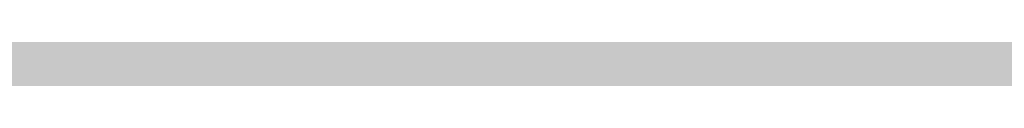
# Model space of a CAD drawing. Units: millimetres. Extents: x 0 to 2267, y 0 to 1823.
# Tile 179 of 256: x 1838.83 to 1841.442, y 1127.306 to 1127.384. Entities that reach past the tile are written whole.
import ezdxf

# ---------------------------------------------------------------- set-up
doc = ezdxf.new("R2010")
doc.units = ezdxf.units.MM
doc.header["$MEASUREMENT"] = 0
doc.layers.add('M-DIMS', color=2, linetype='Continuous', lineweight=25)
doc.layers.add('M-HATC', color=252, linetype='Continuous', lineweight=18)
doc.styles.get("Standard").update_dxf_attribs({"font": 'arial.ttf'})
doc.dimstyles.get("Standard").update_dxf_attribs({"dimtxt": 7, "dimasz": 4, "dimexe": 0.18, "dimexo": 0.0625, "dimgap": 0.09, "dimtad": 0, "dimdec": 0, "dimzin": 0, "dimdsep": 46, "dimtxsty": 'Standard', "dimcen": 0.09, "dimadec": 0, "dimazin": 0, "dimtfac": 1, "dimtdec": 0, "dimtofl": 0, "dimtmove": 0, "dimatfit": 3, "dimfxl": 1, "dimtolj": 1, "dimtzin": 0, "dimarcsym": 0})

# ---------------------------------------------------------------- blocks, each defined once
blk = doc.blocks.new('*D1')
at = {"layer": 'Defpoints', "color": 0, "transparency": 16777216}
for p in [(1593.4289, 1127.4171), (1843.4289, 1127.4171), (1843.4289, 955.6278)]:
    blk.add_point(p, dxfattribs=at)
at = {"layer": 'M-DIMS', "color": 0, "lineweight": -2, "transparency": 16777216}
for p, q in [((1593.4289, 1127.3546), (1593.4289, 955.4478)), ((1843.4289, 1127.3546), (1843.4289, 955.4478)), ((1597.4289, 955.6278), (1710.5582, 955.6278)), ((1839.4289, 955.6278), (1726.2996, 955.6278))]:
    blk.add_line(p, q, dxfattribs=at)
at = {"layer": 'M-DIMS', "color": 0, "transparency": 16777216}
for points in [[(1597.4289, 956.2944), (1597.4289, 954.9611), (1593.4289, 955.6278)], [(1839.4289, 956.2944), (1839.4289, 954.9611), (1843.4289, 955.6278)]]:
    blk.add_solid(points, dxfattribs=at)
at = {"layer": 'M-DIMS', "color": 0, "transparency": 16777216, "insert": (1718.4289, 955.6278), "char_height": 7, "attachment_point": 5}
blk.add_mtext('\\A1;250', dxfattribs=at)

msp = doc.modelspace()

# ---------------------------------------------------------------- hatches: boundary and pattern name
at = {"layer": 'M-HATC'}
h = msp.add_hatch(color=256, dxfattribs=at)
h.dxf.hatch_style = 1
h.paths.add_polyline_path([(2055.771, 1603.062), (1381.0868, 1603.062), (1381.0868, 1598.062), (2055.771, 1598.062)])
h.paths.add_polyline_path([(2055.771, 1598.062), (1381.0868, 1598.062), (1381.0868, 1593.062), (2055.771, 1593.062)])
h.paths.add_polyline_path([(2051.3074, 1536.7609), (1385.5504, 1536.7609), (1385.5504, 1526.7609), (1387.5504, 1526.7609), (1388.5366, 1525.0528), (1385.3319, 1521.2335), (1385.3319, 1521.2226), (2050.2542, 1522.7491), (2048.3212, 1525.0528), (2049.3074, 1526.7609), (2051.3074, 1526.7609)])
edge = h.paths.add_edge_path()
edge.add_arc((1847.5345, 1379.1492), 135, 222.603061, 222.890851, ccw=False)
edge.add_line((1748.1663, 1287.7656), (1683.0921, 1287.7656))
edge.add_arc((1583.7239, 1379.1492), 135, 317.109149, 317.396939, ccw=False)
edge.add_arc((1678.9686, 1290.6707), 5, 222.8909, 317.1091, ccw=False)
edge.add_arc((1774.2133, 1379.1492), 135, 222.603061, 222.890851, ccw=False)
edge.add_line((1674.8451, 1287.7656), (1609.7709, 1287.7656))
edge.add_arc((1510.4027, 1379.1492), 135, 317.109149, 317.396939, ccw=False)
edge.add_arc((1605.6474, 1290.6707), 5, 222.8909, 317.1091, ccw=False)
edge.add_arc((1700.8921, 1379.1492), 135, 222.603061, 222.890851, ccw=False)
edge.add_line((1601.5239, 1287.7656), (1536.4497, 1287.7656))
edge.add_arc((1437.0815, 1379.1492), 135, 317.109149, 317.396939, ccw=False)
edge.add_arc((1532.3262, 1290.6707), 5, 222.8909, 317.1091, ccw=False)
edge.add_arc((1627.5709, 1379.1492), 135, 222.603061, 222.890851, ccw=False)
edge.add_line((1528.2027, 1287.7656), (1505.9289, 1287.7656))
edge.add_spline(control_points=[(1505.9289, 1287.7656), (1504.2622, 1287.7656), (1504.2622, 1282.7656), (1505.9289, 1282.7656)], knot_values=[0, 0, 0, 0, 5, 5, 5, 5], degree=3, periodic=0)
edge.add_line((1505.9289, 1282.7656), (1930.9289, 1282.7656))
edge.add_spline(control_points=[(1930.9289, 1282.7656), (1932.5956, 1282.7656), (1932.5956, 1287.7656), (1930.9289, 1287.7656)], knot_values=[0, 0, 0, 0, 5, 5, 5, 5], degree=3, periodic=0)
edge.add_line((1930.9289, 1287.7656), (1903.0557, 1287.7656))
edge.add_arc((1803.6875, 1379.1492), 135, 317.109149, 317.396939, ccw=False)
edge.add_arc((1898.9322, 1290.6707), 5, 222.8909, 317.1091, ccw=False)
edge.add_arc((1994.1769, 1379.1492), 135, 222.603061, 222.890851, ccw=False)
edge.add_line((1894.8087, 1287.7656), (1829.7345, 1287.7656))
edge.add_arc((1730.3663, 1379.1492), 135, 317.109149, 317.396939, ccw=False)
edge.add_arc((1825.611, 1290.6707), 5, 222.8909, 317.1091, ccw=False)
edge.add_arc((1920.8557, 1379.1492), 135, 222.603061, 222.890851, ccw=False)
edge.add_line((1821.4875, 1287.7656), (1756.4133, 1287.7656))
edge.add_arc((1657.0451, 1379.1492), 135, 317.109149, 317.396939, ccw=False)
edge.add_arc((1752.2898, 1290.6707), 5, 222.8909, 317.1091, ccw=False)
edge = h.paths.add_edge_path()
edge.add_spline(control_points=[(1843.4289, 1227.2475), (1845.0956, 1227.2475), (1845.0956, 1232.2475), (1843.4289, 1232.2475)], knot_values=[0, 0, 0, 0, 5, 5, 5, 5], degree=3, periodic=0)
edge.add_line((1843.4289, 1232.2475), (1593.4289, 1232.2475))
edge.add_spline(control_points=[(1593.4289, 1232.2475), (1591.7622, 1232.2475), (1591.7622, 1227.2475), (1593.4289, 1227.2475)], knot_values=[0, 0, 0, 0, 5, 5, 5, 5], degree=3, periodic=0)
edge.add_line((1593.4289, 1227.2475), (1843.4289, 1227.2475))
h.paths.add_polyline_path([(1905.9289, 1127.4171), (1530.9289, 1127.4171, 0.414214), (1520.9289, 1117.4171), (1530.9289, 1117.4171), (1915.9289, 1117.4171, 0.414214)])
edge = h.paths.add_edge_path()
edge.add_arc((1397.0858, 1498.4078), 12.7299, 90.78215, 190.87871, ccw=False)
edge.add_line((1396.912, 1511.1365), (1428.0097, 1511.3488))
edge.add_line((1428.0097, 1511.3488), (1433.0097, 1511.3488))
edge.add_line((1433.0097, 1511.3488), (1434.439, 1511.3488))
edge.add_arc((1419.474, 1498.0804), 20, 41.561, 74.08211)
edge.add_line((1424.9592, 1517.3135), (1399.9351, 1517.2561))
edge.add_spline(control_points=[(1399.9307, 1517.2561), (1399.884, 1517.2131), (1399.8328, 1517.1689), (1399.7774, 1517.1236)], knot_values=[11.567499, 11.567499, 11.567499, 11.567499, 11.814249, 11.814249, 11.814249, 11.814249], degree=3, periodic=0)
edge.add_spline(control_points=[(1399.6328, 1517.0099), (1399.5831, 1516.9721), (1399.5307, 1516.9338), (1399.4759, 1516.8947)], knot_values=[11.167718, 11.167718, 11.167718, 11.167718, 11.365188, 11.365188, 11.365188, 11.365188], degree=3, periodic=0)
edge.add_spline(control_points=[(1399.3398, 1516.8001), (1399.1514, 1516.6719), (1398.9384, 1516.5377), (1398.704, 1516.3994)], knot_values=[10.376405, 10.376405, 10.376405, 10.376405, 11.00994, 11.00994, 11.00994, 11.00994], degree=3, periodic=0)
edge.add_spline(control_points=[(1398.6572, 1516.3719), (1398.5789, 1516.326), (1398.4983, 1516.2797), (1398.4155, 1516.2331)], knot_values=[10.125175, 10.125175, 10.125175, 10.125175, 10.334406, 10.334406, 10.334406, 10.334406], degree=3, periodic=0)
edge.add_spline(control_points=[(1398.2642, 1516.1487), (1398.196, 1516.1111), (1398.1263, 1516.0732), (1398.0555, 1516.0351)], knot_values=[9.832246, 9.832246, 9.832246, 9.832246, 9.999658, 9.999658, 9.999658, 9.999658], degree=3, periodic=0)
edge.add_spline(control_points=[(1397.9987, 1516.0048), (1397.7312, 1515.8621), (1397.446, 1515.7171), (1397.1466, 1515.5714)], knot_values=[9.161808, 9.161808, 9.161808, 9.161808, 9.787769, 9.787769, 9.787769, 9.787769], degree=3, periodic=0)
edge.add_spline(control_points=[(1397.1466, 1515.5714), (1396.8418, 1515.423), (1396.5222, 1515.274), (1396.1914, 1515.1262)], knot_values=[8.524455, 8.524455, 8.524455, 8.524455, 9.161808, 9.161808, 9.161808, 9.161808], degree=3, periodic=0)
edge.add_spline(control_points=[(1396.0777, 1515.0756), (1395.9854, 1515.0348), (1395.8922, 1514.994), (1395.7983, 1514.9534)], knot_values=[8.275193, 8.275193, 8.275193, 8.275193, 8.451726, 8.451726, 8.451726, 8.451726], degree=3, periodic=0)
edge.add_spline(control_points=[(1395.6018, 1514.8691), (1395.4997, 1514.8257), (1395.3968, 1514.7824), (1395.2932, 1514.7394)], knot_values=[7.962917, 7.962917, 7.962917, 7.962917, 8.152764, 8.152764, 8.152764, 8.152764], degree=3, periodic=0)
edge.add_spline(control_points=[(1395.2116, 1514.7057), (1394.8278, 1514.5475), (1394.4345, 1514.3929), (1394.0364, 1514.2442)], knot_values=[7.21254, 7.21254, 7.21254, 7.21254, 7.913148, 7.913148, 7.913148, 7.913148], degree=3, periodic=0)
edge.add_spline(control_points=[(1394.0364, 1514.2442), (1393.7076, 1514.1214), (1393.3754, 1514.0027), (1393.0427, 1513.8895)], knot_values=[6.633733, 6.633733, 6.633733, 6.633733, 7.21254, 7.21254, 7.21254, 7.21254], degree=3, periodic=0)
edge.add_spline(control_points=[(1392.8214, 1513.815), (1392.7198, 1513.7812), (1392.6181, 1513.7479), (1392.5166, 1513.7152)], knot_values=[6.328796, 6.328796, 6.328796, 6.328796, 6.505493, 6.505493, 6.505493, 6.505493], degree=3, periodic=0)
edge.add_spline(control_points=[(1392.5166, 1513.7152), (1392.3187, 1513.6515), (1392.1212, 1513.59), (1391.9244, 1513.531)], knot_values=[5.984605, 5.984605, 5.984605, 5.984605, 6.328796, 6.328796, 6.328796, 6.328796], degree=3, periodic=0)
edge.add_spline(control_points=[(1391.7915, 1513.4915), (1391.3122, 1513.3501), (1390.8384, 1513.2239), (1390.3784, 1513.1171)], knot_values=[5.066697, 5.066697, 5.066697, 5.066697, 5.907055, 5.907055, 5.907055, 5.907055], degree=3, periodic=0)
edge.add_spline(control_points=[(1390.3784, 1513.1171), (1390.1797, 1513.071), (1389.9836, 1513.0284), (1389.7907, 1512.9899)], knot_values=[4.70367, 4.70367, 4.70367, 4.70367, 5.066695, 5.066695, 5.066695, 5.066695], degree=3, periodic=0)
edge.add_spline(control_points=[(1389.422, 1512.9204), (1389.2459, 1512.8892), (1389.0729, 1512.8617), (1388.9036, 1512.8381)], knot_values=[4.130571, 4.130571, 4.130571, 4.130571, 4.469816, 4.469816, 4.469816, 4.469816], degree=3, periodic=0)
edge.add_spline(control_points=[(1388.9036, 1512.8381), (1388.591, 1512.7946), (1388.2911, 1512.7644), (1388.0071, 1512.7494)], knot_values=[3.504031, 3.504031, 3.504031, 3.504031, 4.130571, 4.130571, 4.130571, 4.130571], degree=3, periodic=0)
edge.add_spline(control_points=[(1387.9356, 1512.7459), (1387.8538, 1512.7423), (1387.7733, 1512.74), (1387.6944, 1512.739)], knot_values=[3.268866, 3.268866, 3.268866, 3.268866, 3.451164, 3.451164, 3.451164, 3.451164], degree=3, periodic=0)
edge.add_spline(control_points=[(1387.3351, 1512.7443), (1387.2076, 1512.7499), (1387.0847, 1512.7597), (1386.967, 1512.7739)], knot_values=[2.670686, 2.670686, 2.670686, 2.670686, 2.984, 2.984, 2.984, 2.984], degree=3, periodic=0)
edge.add_spline(control_points=[(1386.8327, 1512.7922), (1386.8209, 1512.7941), (1386.8092, 1512.7959), (1386.7975, 1512.7979)], knot_values=[2.516981, 2.516981, 2.516981, 2.516981, 2.549528, 2.549528, 2.549528, 2.549528], degree=3, periodic=0)
edge.add_spline(control_points=[(1386.4526, 1512.8735), (1386.4257, 1512.881), (1386.3993, 1512.889), (1386.3733, 1512.8972)], knot_values=[2.095869, 2.095869, 2.095869, 2.095869, 2.17941, 2.17941, 2.17941, 2.17941], degree=3, periodic=0)
edge.add_spline(control_points=[(1386.0691, 1513.0189), (1386.0634, 1513.0217), (1386.0577, 1513.0246), (1386.052, 1513.0275)], knot_values=[1.72453, 1.72453, 1.72453, 1.72453, 1.745933, 1.745933, 1.745933, 1.745933], degree=3, periodic=0)
edge.add_arc((1399.474, 1498.0804), 20, 131.82432, 180)
edge.add_arc((1630.3336, 1505.5484), 250.9708, 181.705176, 236.427975)
edge.add_arc((1605.3399, 1483.3044), 218.7822, 238.660829, 243.34961)
edge.add_arc((1647.0911, 1510.3592), 262.8986, 183.129836, 237.853442, ccw=False)
h.paths.add_polyline_path([(1406.5369, 1391.9644, 0.149382), (1491.5506, 1296.4418, -0.129517)], flags=17)
edge = h.paths.add_edge_path()
edge.add_arc((2037.3838, 1498.0804), 20, 0, 48.26587)
edge.add_spline(control_points=[(2050.6973, 1513.0052), (2050.6512, 1512.9847), (2050.6034, 1512.9655), (2050.5539, 1512.9477)], knot_values=[1.835652, 1.835652, 1.835652, 1.835652, 2.000781, 2.000781, 2.000781, 2.000781], degree=3, periodic=0)
edge.add_spline(control_points=[(2050.4616, 1512.9166), (2050.479, 1512.9221), (2050.4963, 1512.9277), (2050.5133, 1512.9335)], knot_values=[2.045477, 2.045477, 2.045477, 2.045477, 2.101389, 2.101389, 2.101389, 2.101389], degree=3, periodic=0)
edge.add_spline(control_points=[(2050.129, 1512.8342), (2050.1984, 1512.8473), (2050.2657, 1512.8623), (2050.3308, 1512.8792)], knot_values=[2.237629, 2.237629, 2.237629, 2.237629, 2.435841, 2.435841, 2.435841, 2.435841], degree=3, periodic=0)
edge.add_spline(control_points=[(2050.0946, 1512.8278), (2050.1061, 1512.8299), (2050.1176, 1512.832), (2050.129, 1512.8342)], knot_values=[2.435841, 2.435841, 2.435841, 2.435841, 2.468321, 2.468321, 2.468321, 2.468321], degree=3, periodic=0)
edge.add_spline(control_points=[(2049.7843, 1512.7851), (2049.8552, 1512.7922), (2049.9243, 1512.8008), (2049.9917, 1512.8109)], knot_values=[2.563852, 2.563852, 2.563852, 2.563852, 2.748541, 2.748541, 2.748541, 2.748541], degree=3, periodic=0)
edge.add_spline(control_points=[(2049.4052, 1512.7617), (2049.5364, 1512.7653), (2049.6629, 1512.773), (2049.7843, 1512.7851)], knot_values=[2.748541, 2.748541, 2.748541, 2.748541, 3.064882, 3.064882, 3.064882, 3.064882], degree=3, periodic=0)
edge.add_spline(control_points=[(2049.1698, 1512.7597), (2049.2336, 1512.7591), (2049.2965, 1512.7594), (2049.3584, 1512.7606)], knot_values=[3.102309, 3.102309, 3.102309, 3.102309, 3.2503, 3.2503, 3.2503, 3.2503], degree=3, periodic=0)
edge.add_spline(control_points=[(2048.8573, 1512.7691), (2048.9638, 1512.7638), (2049.068, 1512.7606), (2049.1698, 1512.7597)], knot_values=[3.2503, 3.2503, 3.2503, 3.2503, 3.486069, 3.486069, 3.486069, 3.486069], degree=3, periodic=0)
edge.add_spline(control_points=[(2048.6924, 1512.7789), (2048.3729, 1512.8009), (2048.0345, 1512.8411), (2047.6817, 1512.897)], knot_values=[3.606429, 3.606429, 3.606429, 3.606429, 4.2989, 4.2989, 4.2989, 4.2989], degree=3, periodic=0)
edge.add_spline(control_points=[(2047.6817, 1512.897), (2047.5458, 1512.9185), (2047.4077, 1512.9424), (2047.2678, 1512.9685)], knot_values=[4.2989, 4.2989, 4.2989, 4.2989, 4.565769, 4.565769, 4.565769, 4.565769], degree=3, periodic=0)
edge.add_spline(control_points=[(2047.2678, 1512.9685), (2047.1449, 1512.9914), (2047.0207, 1513.016), (2046.8951, 1513.0422)], knot_values=[4.565769, 4.565769, 4.565769, 4.565769, 4.799971, 4.799971, 4.799971, 4.799971], degree=3, periodic=0)
edge.add_spline(control_points=[(2046.8951, 1513.0422), (2046.5286, 1513.1188), (2046.1513, 1513.209), (2045.7676, 1513.3107)], knot_values=[4.799971, 4.799971, 4.799971, 4.799971, 5.483718, 5.483718, 5.483718, 5.483718], degree=3, periodic=0)
edge.add_spline(control_points=[(2045.7676, 1513.3107), (2045.3724, 1513.4154), (2044.9704, 1513.5322), (2044.5662, 1513.6588)], knot_values=[5.483718, 5.483718, 5.483718, 5.483718, 6.187866, 6.187866, 6.187866, 6.187866], degree=3, periodic=0)
edge.add_spline(control_points=[(2044.5662, 1513.6588), (2044.4149, 1513.7061), (2044.2633, 1513.7549), (2044.1116, 1513.8048)], knot_values=[6.187866, 6.187866, 6.187866, 6.187866, 6.451551, 6.451551, 6.451551, 6.451551], degree=3, periodic=0)
edge.add_spline(control_points=[(2044.1116, 1513.8048), (2043.9967, 1513.8427), (2043.8817, 1513.8813), (2043.7668, 1513.9205)], knot_values=[6.451551, 6.451551, 6.451551, 6.451551, 6.651434, 6.651434, 6.651434, 6.651434], degree=3, periodic=0)
edge.add_spline(control_points=[(2043.7668, 1513.9205), (2043.3716, 1514.0554), (2042.9774, 1514.1979), (2042.5886, 1514.3458)], knot_values=[6.651434, 6.651434, 6.651434, 6.651434, 7.338879, 7.338879, 7.338879, 7.338879], degree=3, periodic=0)
edge.add_spline(control_points=[(2042.5886, 1514.3458), (2042.1643, 1514.5071), (2041.7465, 1514.6749), (2041.3409, 1514.846)], knot_values=[7.338879, 7.338879, 7.338879, 7.338879, 8.089209, 8.089209, 8.089209, 8.089209], degree=3, periodic=0)
edge.add_spline(control_points=[(2041.3409, 1514.846), (2041.1028, 1514.9465), (2040.869, 1515.0481), (2040.6405, 1515.1502)], knot_values=[8.089209, 8.089209, 8.089209, 8.089209, 8.529587, 8.529587, 8.529587, 8.529587], degree=3, periodic=0)
edge.add_spline(control_points=[(2040.51, 1515.2089), (2040.0824, 1515.4022), (2039.6747, 1515.5971), (2039.295, 1515.7894)], knot_values=[8.613818, 8.613818, 8.613818, 8.613818, 9.44571, 9.44571, 9.44571, 9.44571], degree=3, periodic=0)
edge.add_spline(control_points=[(2039.295, 1515.7894), (2039.0618, 1515.9075), (2038.8391, 1516.0246), (2038.6288, 1516.1398)], knot_values=[9.44571, 9.44571, 9.44571, 9.44571, 9.956404, 9.956404, 9.956404, 9.956404], degree=3, periodic=0)
edge.add_spline(control_points=[(2038.6288, 1516.1398), (2038.5187, 1516.2001), (2038.4121, 1516.2598), (2038.309, 1516.3189)], knot_values=[9.956404, 9.956404, 9.956404, 9.956404, 10.223542, 10.223542, 10.223542, 10.223542], degree=3, periodic=0)
edge.add_spline(control_points=[(2038.309, 1516.3189), (2038.2138, 1516.3735), (2038.1216, 1516.4276), (2038.0328, 1516.481)], knot_values=[10.223542, 10.223542, 10.223542, 10.223542, 10.47051, 10.47051, 10.47051, 10.47051], degree=3, periodic=0)
edge.add_spline(control_points=[(2038.0328, 1516.481), (2037.7855, 1516.6296), (2037.5639, 1516.773), (2037.3722, 1516.909)], knot_values=[10.47051, 10.47051, 10.47051, 10.47051, 11.15767, 11.15767, 11.15767, 11.15767], degree=3, periodic=0)
edge.add_spline(control_points=[(2037.3722, 1516.909), (2037.2789, 1516.9752), (2037.1927, 1517.0396), (2037.1142, 1517.102)], knot_values=[11.15767, 11.15767, 11.15767, 11.15767, 11.49227, 11.49227, 11.49227, 11.49227], degree=3, periodic=0)
edge.add_spline(control_points=[(2036.8564, 1517.3259), (2036.9148, 1517.2692), (2036.9814, 1517.2103), (2037.0557, 1517.1492)], knot_values=[11.577341, 11.577341, 11.577341, 11.577341, 11.91035, 11.91035, 11.91035, 11.91035], degree=3, periodic=0)
edge.add_spline(control_points=[(2036.8074, 1517.3748), (2036.823, 1517.3587), (2036.8393, 1517.3424), (2036.8564, 1517.3259)], knot_values=[11.91035, 11.91035, 11.91035, 11.91035, 12.007402, 12.007402, 12.007402, 12.007402], degree=3, periodic=0)
edge.add_spline(control_points=[(2036.7017, 1517.494), (2036.7104, 1517.483), (2036.7196, 1517.4719), (2036.7291, 1517.4606)], knot_values=[12.184155, 12.184155, 12.184155, 12.184155, 12.255409, 12.255409, 12.255409, 12.255409], degree=3, periodic=0)
edge.add_spline(control_points=[(2036.6159, 1517.6205), (2036.62, 1517.613), (2036.6243, 1517.6055), (2036.6289, 1517.5979)], knot_values=[12.487913, 12.487913, 12.487913, 12.487913, 12.541035, 12.541035, 12.541035, 12.541035], degree=3, periodic=0)
edge.add_spline(control_points=[(2036.5635, 1517.786), (2036.5637, 1517.7794), (2036.5642, 1517.7726), (2036.565, 1517.7658)], knot_values=[12.911761, 12.911761, 12.911761, 12.911761, 12.968286, 12.968286, 12.968286, 12.968286], degree=3, periodic=0)
edge.add_spline(control_points=[(2036.6166, 1517.9304), (2036.6125, 1517.9259), (2036.6086, 1517.9212), (2036.6049, 1517.9165)], knot_values=[13.382527, 13.382527, 13.382527, 13.382527, 13.433791, 13.433791, 13.433791, 13.433791], degree=3, periodic=0)
edge.add_spline(control_points=[(2036.749, 1518.017), (2036.7361, 1518.0116), (2036.7239, 1518.006), (2036.7124, 1518.0002)], knot_values=[13.726299, 13.726299, 13.726299, 13.726299, 13.809928, 13.809928, 13.809928, 13.809928], degree=3, periodic=0)
edge.add_spline(control_points=[(2036.8604, 1518.0528), (2036.8386, 1518.0474), (2036.8181, 1518.0416), (2036.7988, 1518.0353)], knot_values=[13.910887, 13.910887, 13.910887, 13.910887, 14.02153, 14.02153, 14.02153, 14.02153], degree=3, periodic=0)
edge.add_line((2036.9639, 1518.0804), (2032.3838, 1518.0804))
edge.add_line((2032.3838, 1518.0804), (2027.3838, 1518.0804))
edge.add_line((2027.3838, 1518.0804), (2022.3838, 1518.0804))
edge.add_line((2022.3838, 1518.0804), (2017.3838, 1518.0804))
edge.add_arc((2017.3838, 1498.0804), 20, 90, 138.439)
edge.add_line((2002.4188, 1511.3488), (2003.8481, 1511.3488))
edge.add_line((2003.8481, 1511.3488), (2008.8481, 1511.3488))
edge.add_line((2008.8481, 1511.3488), (2039.772, 1511.1377))
edge.add_arc((2039.772, 1498.4078), 12.7299, -10.87871, 90, ccw=False)
edge.add_arc((1789.7668, 1510.3592), 262.8986, 302.146558, 356.870164, ccw=False)
edge.add_arc((1831.5179, 1483.3044), 218.7822, 296.65039, 301.339171)
edge.add_arc((1806.5242, 1505.5484), 250.9708, 303.572025, 358.294824)
h.paths.add_polyline_path([(2030.321, 1391.9644, -0.129517), (1945.3072, 1296.4418, 0.149382)], flags=17)
edge = h.paths.add_edge_path()
edge.add_spline(control_points=[(2037.2464, 1518.0821), (2037.2898, 1518.081), (2037.3355, 1518.0804), (2037.3838, 1518.0804)], knot_values=[0.000012, 0.000012, 0.000012, 0.000012, 0.144754, 0.144754, 0.144754, 0.144754], degree=3, periodic=0)
edge.add_line((2037.3357, 1518.0804), (2037.0096, 1518.0804))
edge.add_spline(control_points=[(2037.0096, 1518.0804), (2036.9822, 1518.0768), (2036.956, 1518.0727), (2036.9312, 1518.0681)], knot_values=[14.13465, 14.13465, 14.13465, 14.13465, 14.247197, 14.247197, 14.247197, 14.247197], degree=3, periodic=0)
edge.add_spline(control_points=[(2036.9312, 1518.0681), (2036.9276, 1518.0674), (2036.9241, 1518.0667), (2036.9205, 1518.0661)], knot_values=[14.118315, 14.118315, 14.118315, 14.118315, 14.13465, 14.13465, 14.13465, 14.13465], degree=3, periodic=0)
edge.add_spline(control_points=[(2036.9205, 1518.0661), (2036.9118, 1518.0644), (2036.9032, 1518.0626), (2036.8948, 1518.0608)], knot_values=[14.078086, 14.078086, 14.078086, 14.078086, 14.118315, 14.118315, 14.118315, 14.118315], degree=3, periodic=0)
edge.add_spline(control_points=[(2036.8948, 1518.0608), (2036.883, 1518.0583), (2036.8716, 1518.0556), (2036.8604, 1518.0528)], knot_values=[14.02153, 14.02153, 14.02153, 14.02153, 14.078086, 14.078086, 14.078086, 14.078086], degree=3, periodic=0)
edge.add_spline(control_points=[(2036.8604, 1518.0528), (2036.8386, 1518.0474), (2036.8181, 1518.0416), (2036.7988, 1518.0353)], knot_values=[13.910887, 13.910887, 13.910887, 13.910887, 14.02153, 14.02153, 14.02153, 14.02153], degree=3, periodic=0)
edge.add_spline(control_points=[(2036.7988, 1518.0353), (2036.7981, 1518.035), (2036.7974, 1518.0348), (2036.7967, 1518.0346)], knot_values=[13.906906, 13.906906, 13.906906, 13.906906, 13.910887, 13.910887, 13.910887, 13.910887], degree=3, periodic=0)
edge.add_spline(control_points=[(2036.7967, 1518.0346), (2036.7882, 1518.0318), (2036.7799, 1518.0289), (2036.7719, 1518.0259)], knot_values=[13.857826, 13.857826, 13.857826, 13.857826, 13.906906, 13.906906, 13.906906, 13.906906], degree=3, periodic=0)
edge.add_spline(control_points=[(2036.7719, 1518.0259), (2036.764, 1518.023), (2036.7564, 1518.02), (2036.749, 1518.017)], knot_values=[13.809928, 13.809928, 13.809928, 13.809928, 13.857826, 13.857826, 13.857826, 13.857826], degree=3, periodic=0)
edge.add_spline(control_points=[(2036.749, 1518.017), (2036.7361, 1518.0116), (2036.7239, 1518.006), (2036.7124, 1518.0002)], knot_values=[13.726299, 13.726299, 13.726299, 13.726299, 13.809928, 13.809928, 13.809928, 13.809928], degree=3, periodic=0)
edge.add_spline(control_points=[(2036.7124, 1518.0002), (2036.7121, 1518), (2036.7118, 1517.9999), (2036.7115, 1517.9997)], knot_values=[13.723993, 13.723993, 13.723993, 13.723993, 13.726299, 13.726299, 13.726299, 13.726299], degree=3, periodic=0)
edge.add_spline(control_points=[(2036.7115, 1517.9997), (2036.7063, 1517.9971), (2036.7013, 1517.9944), (2036.6965, 1517.9917)], knot_values=[13.686536, 13.686536, 13.686536, 13.686536, 13.723993, 13.723993, 13.723993, 13.723993], degree=3, periodic=0)
edge.add_spline(control_points=[(2036.6965, 1517.9917), (2036.6919, 1517.9891), (2036.6874, 1517.9865), (2036.6831, 1517.9839)], knot_values=[13.651251, 13.651251, 13.651251, 13.651251, 13.686536, 13.686536, 13.686536, 13.686536], degree=3, periodic=0)
edge.add_spline(control_points=[(2036.6831, 1517.9839), (2036.6764, 1517.9798), (2036.67, 1517.9757), (2036.6639, 1517.9714)], knot_values=[13.596804, 13.596804, 13.596804, 13.596804, 13.651251, 13.651251, 13.651251, 13.651251], degree=3, periodic=0)
edge.add_spline(control_points=[(2036.6639, 1517.9714), (2036.6636, 1517.9712), (2036.6633, 1517.9709), (2036.6629, 1517.9707)], knot_values=[13.593956, 13.593956, 13.593956, 13.593956, 13.596804, 13.596804, 13.596804, 13.596804], degree=3, periodic=0)
edge.add_spline(control_points=[(2036.6629, 1517.9707), (2036.6603, 1517.9689), (2036.6577, 1517.967), (2036.6552, 1517.9651)], knot_values=[13.570322, 13.570322, 13.570322, 13.570322, 13.593956, 13.593956, 13.593956, 13.593956], degree=3, periodic=0)
edge.add_spline(control_points=[(2036.6552, 1517.9651), (2036.6525, 1517.9631), (2036.6499, 1517.9611), (2036.6474, 1517.9591)], knot_values=[13.545477, 13.545477, 13.545477, 13.545477, 13.570322, 13.570322, 13.570322, 13.570322], degree=3, periodic=0)
edge.add_spline(control_points=[(2036.6474, 1517.9591), (2036.6472, 1517.9589), (2036.6471, 1517.9588), (2036.6469, 1517.9587)], knot_values=[13.543931, 13.543931, 13.543931, 13.543931, 13.545477, 13.545477, 13.545477, 13.545477], degree=3, periodic=0)
edge.add_spline(control_points=[(2036.6469, 1517.9587), (2036.6412, 1517.9541), (2036.6358, 1517.9494), (2036.6307, 1517.9447)], knot_values=[13.488237, 13.488237, 13.488237, 13.488237, 13.543931, 13.543931, 13.543931, 13.543931], degree=3, periodic=0)
edge.add_spline(control_points=[(2036.6307, 1517.9447), (2036.6282, 1517.9423), (2036.6257, 1517.9399), (2036.6233, 1517.9374)], knot_values=[13.460307, 13.460307, 13.460307, 13.460307, 13.488237, 13.488237, 13.488237, 13.488237], degree=3, periodic=0)
edge.add_spline(control_points=[(2036.6233, 1517.9374), (2036.6215, 1517.9356), (2036.6198, 1517.9338), (2036.6181, 1517.932)], knot_values=[13.439712, 13.439712, 13.439712, 13.439712, 13.460307, 13.460307, 13.460307, 13.460307], degree=3, periodic=0)
edge.add_spline(control_points=[(2036.6181, 1517.932), (2036.6176, 1517.9315), (2036.6171, 1517.9309), (2036.6166, 1517.9304)], knot_values=[13.433791, 13.433791, 13.433791, 13.433791, 13.439712, 13.439712, 13.439712, 13.439712], degree=3, periodic=0)
edge.add_spline(control_points=[(2036.6166, 1517.9304), (2036.6125, 1517.9259), (2036.6086, 1517.9212), (2036.6049, 1517.9165)], knot_values=[13.382527, 13.382527, 13.382527, 13.382527, 13.433791, 13.433791, 13.433791, 13.433791], degree=3, periodic=0)
edge.add_spline(control_points=[(2036.6049, 1517.9165), (2036.6026, 1517.9135), (2036.6004, 1517.9104), (2036.5982, 1517.9074)], knot_values=[13.350017, 13.350017, 13.350017, 13.350017, 13.382527, 13.382527, 13.382527, 13.382527], degree=3, periodic=0)
edge.add_spline(control_points=[(2036.5982, 1517.9074), (2036.5972, 1517.9059), (2036.5962, 1517.9043), (2036.5952, 1517.9028)], knot_values=[13.333922, 13.333922, 13.333922, 13.333922, 13.350017, 13.350017, 13.350017, 13.350017], degree=3, periodic=0)
edge.add_spline(control_points=[(2036.5952, 1517.9028), (2036.5945, 1517.9018), (2036.5939, 1517.9009), (2036.5933, 1517.8999)], knot_values=[13.323828, 13.323828, 13.323828, 13.323828, 13.333922, 13.333922, 13.333922, 13.333922], degree=3, periodic=0)
edge.add_spline(control_points=[(2036.5933, 1517.8999), (2036.5905, 1517.8955), (2036.5879, 1517.8909), (2036.5855, 1517.8864)], knot_values=[13.277545, 13.277545, 13.277545, 13.277545, 13.323828, 13.323828, 13.323828, 13.323828], degree=3, periodic=0)
edge.add_spline(control_points=[(2036.5855, 1517.8864), (2036.5836, 1517.8827), (2036.5817, 1517.8789), (2036.5801, 1517.8751)], knot_values=[13.240119, 13.240119, 13.240119, 13.240119, 13.277545, 13.277545, 13.277545, 13.277545], degree=3, periodic=0)
edge.add_spline(control_points=[(2036.5801, 1517.8751), (2036.5795, 1517.8739), (2036.579, 1517.8727), (2036.5785, 1517.8715)], knot_values=[13.228211, 13.228211, 13.228211, 13.228211, 13.240119, 13.240119, 13.240119, 13.240119], degree=3, periodic=0)
edge.add_spline(control_points=[(2036.5785, 1517.8715), (2036.578, 1517.8702), (2036.5774, 1517.869), (2036.5769, 1517.8677)], knot_values=[13.215717, 13.215717, 13.215717, 13.215717, 13.228211, 13.228211, 13.228211, 13.228211], degree=3, periodic=0)
edge.add_spline(control_points=[(2036.5769, 1517.8677), (2036.5755, 1517.864), (2036.5741, 1517.8603), (2036.5729, 1517.8565)], knot_values=[13.179847, 13.179847, 13.179847, 13.179847, 13.215717, 13.215717, 13.215717, 13.215717], degree=3, periodic=0)
edge.add_spline(control_points=[(2036.5729, 1517.8565), (2036.5713, 1517.8515), (2036.5699, 1517.8464), (2036.5687, 1517.8413)], knot_values=[13.132017, 13.132017, 13.132017, 13.132017, 13.179847, 13.179847, 13.179847, 13.179847], degree=3, periodic=0)
edge.add_spline(control_points=[(2036.5687, 1517.8413), (2036.5684, 1517.8402), (2036.5682, 1517.8392), (2036.568, 1517.8382)], knot_values=[13.122482, 13.122482, 13.122482, 13.122482, 13.132017, 13.132017, 13.132017, 13.132017], degree=3, periodic=0)
edge.add_spline(control_points=[(2036.568, 1517.8382), (2036.5676, 1517.8363), (2036.5672, 1517.8345), (2036.5669, 1517.8327)], knot_values=[13.105592, 13.105592, 13.105592, 13.105592, 13.122482, 13.122482, 13.122482, 13.122482], degree=3, periodic=0)
edge.add_spline(control_points=[(2036.5669, 1517.8327), (2036.5662, 1517.8292), (2036.5657, 1517.8257), (2036.5652, 1517.8222)], knot_values=[13.074063, 13.074063, 13.074063, 13.074063, 13.105592, 13.105592, 13.105592, 13.105592], degree=3, periodic=0)
edge.add_spline(control_points=[(2036.5652, 1517.8222), (2036.5652, 1517.8222), (2036.5652, 1517.8222), (2036.5652, 1517.8222)], knot_values=[13.074043, 13.074043, 13.074043, 13.074043, 13.074063, 13.074063, 13.074063, 13.074063], degree=3, periodic=0)
edge.add_spline(control_points=[(2036.5652, 1517.8222), (2036.5644, 1517.8164), (2036.5639, 1517.8106), (2036.5636, 1517.8046)], knot_values=[13.021884, 13.021884, 13.021884, 13.021884, 13.074043, 13.074043, 13.074043, 13.074043], degree=3, periodic=0)
edge.add_spline(control_points=[(2036.5636, 1517.8046), (2036.5636, 1517.804), (2036.5636, 1517.8034), (2036.5635, 1517.8028)], knot_values=[13.01674, 13.01674, 13.01674, 13.01674, 13.021884, 13.021884, 13.021884, 13.021884], degree=3, periodic=0)
edge.add_spline(control_points=[(2036.5635, 1517.8028), (2036.5634, 1517.8005), (2036.5634, 1517.7982), (2036.5634, 1517.7958)], knot_values=[12.996438, 12.996438, 12.996438, 12.996438, 13.01674, 13.01674, 13.01674, 13.01674], degree=3, periodic=0)
edge.add_spline(control_points=[(2036.5634, 1517.7958), (2036.5633, 1517.7926), (2036.5634, 1517.7893), (2036.5635, 1517.786)], knot_values=[12.968286, 12.968286, 12.968286, 12.968286, 12.996438, 12.996438, 12.996438, 12.996438], degree=3, periodic=0)
edge.add_spline(control_points=[(2036.5635, 1517.786), (2036.5637, 1517.7794), (2036.5642, 1517.7726), (2036.565, 1517.7658)], knot_values=[12.911761, 12.911761, 12.911761, 12.911761, 12.968286, 12.968286, 12.968286, 12.968286], degree=3, periodic=0)
edge.add_spline(control_points=[(2036.565, 1517.7658), (2036.565, 1517.7657), (2036.565, 1517.7656), (2036.565, 1517.7656)], knot_values=[12.911017, 12.911017, 12.911017, 12.911017, 12.911761, 12.911761, 12.911761, 12.911761], degree=3, periodic=0)
edge.add_spline(control_points=[(2036.565, 1517.7656), (2036.5654, 1517.7625), (2036.5658, 1517.7593), (2036.5663, 1517.7562)], knot_values=[12.88528, 12.88528, 12.88528, 12.88528, 12.911017, 12.911017, 12.911017, 12.911017], degree=3, periodic=0)
edge.add_spline(control_points=[(2036.5663, 1517.7562), (2036.5667, 1517.7534), (2036.5672, 1517.7506), (2036.5677, 1517.7478)], knot_values=[12.862519, 12.862519, 12.862519, 12.862519, 12.88528, 12.88528, 12.88528, 12.88528], degree=3, periodic=0)
edge.add_spline(control_points=[(2036.5677, 1517.7478), (2036.5678, 1517.7474), (2036.5679, 1517.7469), (2036.568, 1517.7465)], knot_values=[12.858885, 12.858885, 12.858885, 12.858885, 12.862519, 12.862519, 12.862519, 12.862519], degree=3, periodic=0)
edge.add_spline(control_points=[(2036.568, 1517.7465), (2036.5692, 1517.7399), (2036.5707, 1517.7332), (2036.5724, 1517.7264)], knot_values=[12.8053, 12.8053, 12.8053, 12.8053, 12.858885, 12.858885, 12.858885, 12.858885], degree=3, periodic=0)
edge.add_spline(control_points=[(2036.5724, 1517.7264), (2036.5734, 1517.7226), (2036.5745, 1517.7187), (2036.5756, 1517.7149)], knot_values=[12.775176, 12.775176, 12.775176, 12.775176, 12.8053, 12.8053, 12.8053, 12.8053], degree=3, periodic=0)
edge.add_spline(control_points=[(2036.5756, 1517.7149), (2036.5763, 1517.7125), (2036.577, 1517.7102), (2036.5778, 1517.7078)], knot_values=[12.756759, 12.756759, 12.756759, 12.756759, 12.775176, 12.775176, 12.775176, 12.775176], degree=3, periodic=0)
edge.add_spline(control_points=[(2036.5778, 1517.7078), (2036.5781, 1517.7067), (2036.5784, 1517.7057), (2036.5787, 1517.7047)], knot_values=[12.748742, 12.748742, 12.748742, 12.748742, 12.756759, 12.756759, 12.756759, 12.756759], degree=3, periodic=0)
edge.add_spline(control_points=[(2036.5787, 1517.7047), (2036.5808, 1517.6983), (2036.5831, 1517.6919), (2036.5856, 1517.6854)], knot_values=[12.69959, 12.69959, 12.69959, 12.69959, 12.748742, 12.748742, 12.748742, 12.748742], degree=3, periodic=0)
edge.add_spline(control_points=[(2036.5856, 1517.6854), (2036.5876, 1517.68), (2036.5898, 1517.6746), (2036.5921, 1517.6692)], knot_values=[12.659038, 12.659038, 12.659038, 12.659038, 12.69959, 12.69959, 12.69959, 12.69959], degree=3, periodic=0)
edge.add_spline(control_points=[(2036.5921, 1517.6692), (2036.594, 1517.6648), (2036.5959, 1517.6605), (2036.5979, 1517.6561)], knot_values=[12.626806, 12.626806, 12.626806, 12.626806, 12.659038, 12.659038, 12.659038, 12.659038], degree=3, periodic=0)
edge.add_spline(control_points=[(2036.5979, 1517.6561), (2036.5984, 1517.6551), (2036.5989, 1517.6541), (2036.5993, 1517.6531)], knot_values=[12.619394, 12.619394, 12.619394, 12.619394, 12.626806, 12.626806, 12.626806, 12.626806], degree=3, periodic=0)
edge.add_spline(control_points=[(2036.5993, 1517.6531), (2036.6043, 1517.6424), (2036.6099, 1517.6315), (2036.6159, 1517.6205)], knot_values=[12.541039, 12.541039, 12.541039, 12.541039, 12.619394, 12.619394, 12.619394, 12.619394], degree=3, periodic=0)
edge.add_spline(control_points=[(2036.6159, 1517.6205), (2036.6159, 1517.6205), (2036.6159, 1517.6205), (2036.6159, 1517.6205)], knot_values=[12.541035, 12.541035, 12.541035, 12.541035, 12.541039, 12.541039, 12.541039, 12.541039], degree=3, periodic=0)
edge.add_spline(control_points=[(2036.6159, 1517.6205), (2036.62, 1517.613), (2036.6243, 1517.6055), (2036.6289, 1517.5979)], knot_values=[12.487913, 12.487913, 12.487913, 12.487913, 12.541035, 12.541035, 12.541035, 12.541035], degree=3, periodic=0)
edge.add_spline(control_points=[(2036.6289, 1517.5979), (2036.6326, 1517.5916), (2036.6365, 1517.5853), (2036.6406, 1517.5789)], knot_values=[12.443982, 12.443982, 12.443982, 12.443982, 12.487913, 12.487913, 12.487913, 12.487913], degree=3, periodic=0)
edge.add_spline(control_points=[(2036.6406, 1517.5789), (2036.6414, 1517.5776), (2036.6423, 1517.5763), (2036.6431, 1517.5749)], knot_values=[12.434996, 12.434996, 12.434996, 12.434996, 12.443982, 12.443982, 12.443982, 12.443982], degree=3, periodic=0)
edge.add_spline(control_points=[(2036.6431, 1517.5749), (2036.6531, 1517.5596), (2036.6639, 1517.5439), (2036.6756, 1517.528)], knot_values=[12.329647, 12.329647, 12.329647, 12.329647, 12.434996, 12.434996, 12.434996, 12.434996], degree=3, periodic=0)
edge.add_spline(control_points=[(2036.6756, 1517.528), (2036.6839, 1517.5168), (2036.6925, 1517.5055), (2036.7017, 1517.494)], knot_values=[12.255409, 12.255409, 12.255409, 12.255409, 12.329647, 12.329647, 12.329647, 12.329647], degree=3, periodic=0)
edge.add_spline(control_points=[(2036.7017, 1517.494), (2036.7104, 1517.483), (2036.7196, 1517.4719), (2036.7291, 1517.4606)], knot_values=[12.184155, 12.184155, 12.184155, 12.184155, 12.255409, 12.255409, 12.255409, 12.255409], degree=3, periodic=0)
edge.add_spline(control_points=[(2036.7291, 1517.4606), (2036.7436, 1517.4435), (2036.759, 1517.4262), (2036.7753, 1517.4085)], knot_values=[12.075961, 12.075961, 12.075961, 12.075961, 12.184155, 12.184155, 12.184155, 12.184155], degree=3, periodic=0)
edge.add_spline(control_points=[(2036.7753, 1517.4085), (2036.7763, 1517.4075), (2036.7773, 1517.4064), (2036.7783, 1517.4054)], knot_values=[12.069502, 12.069502, 12.069502, 12.069502, 12.075961, 12.075961, 12.075961, 12.075961], degree=3, periodic=0)
edge.add_spline(control_points=[(2036.7783, 1517.4054), (2036.7877, 1517.3953), (2036.7974, 1517.385), (2036.8074, 1517.3748)], knot_values=[12.007402, 12.007402, 12.007402, 12.007402, 12.069502, 12.069502, 12.069502, 12.069502], degree=3, periodic=0)
edge.add_spline(control_points=[(2036.8074, 1517.3748), (2036.823, 1517.3587), (2036.8393, 1517.3424), (2036.8564, 1517.3259)], knot_values=[11.91035, 11.91035, 11.91035, 11.91035, 12.007402, 12.007402, 12.007402, 12.007402], degree=3, periodic=0)
edge.add_spline(control_points=[(2036.8564, 1517.3259), (2036.9148, 1517.2692), (2036.9814, 1517.2103), (2037.0557, 1517.1492)], knot_values=[11.577341, 11.577341, 11.577341, 11.577341, 11.91035, 11.91035, 11.91035, 11.91035], degree=3, periodic=0)
edge.add_spline(control_points=[(2037.0557, 1517.1492), (2037.0747, 1517.1336), (2037.0942, 1517.1179), (2037.1142, 1517.102)], knot_values=[11.49227, 11.49227, 11.49227, 11.49227, 11.577341, 11.577341, 11.577341, 11.577341], degree=3, periodic=0)
edge.add_spline(control_points=[(2037.1142, 1517.102), (2037.1927, 1517.0396), (2037.2789, 1516.9752), (2037.3722, 1516.909)], knot_values=[11.15767, 11.15767, 11.15767, 11.15767, 11.49227, 11.49227, 11.49227, 11.49227], degree=3, periodic=0)
edge.add_spline(control_points=[(2037.3722, 1516.909), (2037.5639, 1516.773), (2037.7855, 1516.6296), (2038.0328, 1516.481)], knot_values=[10.47051, 10.47051, 10.47051, 10.47051, 11.15767, 11.15767, 11.15767, 11.15767], degree=3, periodic=0)
edge.add_spline(control_points=[(2038.0328, 1516.481), (2038.1216, 1516.4276), (2038.2138, 1516.3735), (2038.309, 1516.3189)], knot_values=[10.223542, 10.223542, 10.223542, 10.223542, 10.47051, 10.47051, 10.47051, 10.47051], degree=3, periodic=0)
edge.add_spline(control_points=[(2038.309, 1516.3189), (2038.4121, 1516.2598), (2038.5187, 1516.2001), (2038.6288, 1516.1398)], knot_values=[9.956404, 9.956404, 9.956404, 9.956404, 10.223542, 10.223542, 10.223542, 10.223542], degree=3, periodic=0)
edge.add_spline(control_points=[(2038.6288, 1516.1398), (2038.8391, 1516.0246), (2039.0618, 1515.9075), (2039.295, 1515.7894)], knot_values=[9.44571, 9.44571, 9.44571, 9.44571, 9.956404, 9.956404, 9.956404, 9.956404], degree=3, periodic=0)
edge.add_spline(control_points=[(2039.295, 1515.7894), (2039.6747, 1515.5971), (2040.0824, 1515.4022), (2040.51, 1515.2089)], knot_values=[8.613818, 8.613818, 8.613818, 8.613818, 9.44571, 9.44571, 9.44571, 9.44571], degree=3, periodic=0)
edge.add_spline(control_points=[(2040.51, 1515.2089), (2040.5533, 1515.1893), (2040.5968, 1515.1697), (2040.6405, 1515.1502)], knot_values=[8.529587, 8.529587, 8.529587, 8.529587, 8.613818, 8.613818, 8.613818, 8.613818], degree=3, periodic=0)
edge.add_spline(control_points=[(2040.6405, 1515.1502), (2040.869, 1515.0481), (2041.1028, 1514.9465), (2041.3409, 1514.846)], knot_values=[8.089209, 8.089209, 8.089209, 8.089209, 8.529587, 8.529587, 8.529587, 8.529587], degree=3, periodic=0)
edge.add_spline(control_points=[(2041.3409, 1514.846), (2041.7465, 1514.6749), (2042.1643, 1514.5071), (2042.5886, 1514.3458)], knot_values=[7.338879, 7.338879, 7.338879, 7.338879, 8.089209, 8.089209, 8.089209, 8.089209], degree=3, periodic=0)
edge.add_spline(control_points=[(2042.5886, 1514.3458), (2042.9774, 1514.1979), (2043.3716, 1514.0554), (2043.7668, 1513.9205)], knot_values=[6.651434, 6.651434, 6.651434, 6.651434, 7.338879, 7.338879, 7.338879, 7.338879], degree=3, periodic=0)
edge.add_spline(control_points=[(2043.7668, 1513.9205), (2043.8817, 1513.8813), (2043.9967, 1513.8427), (2044.1116, 1513.8048)], knot_values=[6.451551, 6.451551, 6.451551, 6.451551, 6.651434, 6.651434, 6.651434, 6.651434], degree=3, periodic=0)
edge.add_spline(control_points=[(2044.1116, 1513.8048), (2044.2633, 1513.7549), (2044.4149, 1513.7061), (2044.5662, 1513.6588)], knot_values=[6.187866, 6.187866, 6.187866, 6.187866, 6.451551, 6.451551, 6.451551, 6.451551], degree=3, periodic=0)
edge.add_spline(control_points=[(2044.5662, 1513.6588), (2044.9704, 1513.5322), (2045.3724, 1513.4154), (2045.7676, 1513.3107)], knot_values=[5.483718, 5.483718, 5.483718, 5.483718, 6.187866, 6.187866, 6.187866, 6.187866], degree=3, periodic=0)
edge.add_spline(control_points=[(2045.7676, 1513.3107), (2046.1513, 1513.209), (2046.5286, 1513.1188), (2046.8951, 1513.0422)], knot_values=[4.799971, 4.799971, 4.799971, 4.799971, 5.483718, 5.483718, 5.483718, 5.483718], degree=3, periodic=0)
edge.add_spline(control_points=[(2046.8951, 1513.0422), (2047.0207, 1513.016), (2047.1449, 1512.9914), (2047.2678, 1512.9685)], knot_values=[4.565769, 4.565769, 4.565769, 4.565769, 4.799971, 4.799971, 4.799971, 4.799971], degree=3, periodic=0)
edge.add_spline(control_points=[(2047.2678, 1512.9685), (2047.4077, 1512.9424), (2047.5458, 1512.9185), (2047.6817, 1512.897)], knot_values=[4.2989, 4.2989, 4.2989, 4.2989, 4.565769, 4.565769, 4.565769, 4.565769], degree=3, periodic=0)
edge.add_spline(control_points=[(2047.6817, 1512.897), (2048.0345, 1512.8411), (2048.3729, 1512.8009), (2048.6924, 1512.7789)], knot_values=[3.606429, 3.606429, 3.606429, 3.606429, 4.2989, 4.2989, 4.2989, 4.2989], degree=3, periodic=0)
edge.add_spline(control_points=[(2048.6924, 1512.7789), (2048.7479, 1512.7751), (2048.8029, 1512.7718), (2048.8573, 1512.7691)], knot_values=[3.486069, 3.486069, 3.486069, 3.486069, 3.606429, 3.606429, 3.606429, 3.606429], degree=3, periodic=0)
edge.add_spline(control_points=[(2048.8573, 1512.7691), (2048.9638, 1512.7638), (2049.068, 1512.7606), (2049.1698, 1512.7597)], knot_values=[3.2503, 3.2503, 3.2503, 3.2503, 3.486069, 3.486069, 3.486069, 3.486069], degree=3, periodic=0)
edge.add_spline(control_points=[(2049.1698, 1512.7597), (2049.2336, 1512.7591), (2049.2965, 1512.7594), (2049.3584, 1512.7606)], knot_values=[3.102309, 3.102309, 3.102309, 3.102309, 3.2503, 3.2503, 3.2503, 3.2503], degree=3, periodic=0)
edge.add_spline(control_points=[(2049.3584, 1512.7606), (2049.3741, 1512.7609), (2049.3897, 1512.7613), (2049.4052, 1512.7617)], knot_values=[3.064882, 3.064882, 3.064882, 3.064882, 3.102309, 3.102309, 3.102309, 3.102309], degree=3, periodic=0)
edge.add_spline(control_points=[(2049.4052, 1512.7617), (2049.5364, 1512.7653), (2049.6629, 1512.773), (2049.7843, 1512.7851)], knot_values=[2.748541, 2.748541, 2.748541, 2.748541, 3.064882, 3.064882, 3.064882, 3.064882], degree=3, periodic=0)
edge.add_spline(control_points=[(2049.7843, 1512.7851), (2049.8552, 1512.7922), (2049.9243, 1512.8008), (2049.9917, 1512.8109)], knot_values=[2.563852, 2.563852, 2.563852, 2.563852, 2.748541, 2.748541, 2.748541, 2.748541], degree=3, periodic=0)
edge.add_spline(control_points=[(2049.9917, 1512.8109), (2050.0265, 1512.8161), (2050.0608, 1512.8218), (2050.0946, 1512.8278)], knot_values=[2.468321, 2.468321, 2.468321, 2.468321, 2.563852, 2.563852, 2.563852, 2.563852], degree=3, periodic=0)
edge.add_spline(control_points=[(2050.0946, 1512.8278), (2050.1061, 1512.8299), (2050.1176, 1512.832), (2050.129, 1512.8342)], knot_values=[2.435841, 2.435841, 2.435841, 2.435841, 2.468321, 2.468321, 2.468321, 2.468321], degree=3, periodic=0)
edge.add_spline(control_points=[(2050.129, 1512.8342), (2050.1984, 1512.8473), (2050.2657, 1512.8623), (2050.3308, 1512.8792)], knot_values=[2.237629, 2.237629, 2.237629, 2.237629, 2.435841, 2.435841, 2.435841, 2.435841], degree=3, periodic=0)
edge.add_spline(control_points=[(2050.3308, 1512.8792), (2050.3754, 1512.8908), (2050.4191, 1512.9032), (2050.4616, 1512.9166)], knot_values=[2.101389, 2.101389, 2.101389, 2.101389, 2.237629, 2.237629, 2.237629, 2.237629], degree=3, periodic=0)
edge.add_spline(control_points=[(2050.4616, 1512.9166), (2050.479, 1512.9221), (2050.4963, 1512.9277), (2050.5133, 1512.9335)], knot_values=[2.045477, 2.045477, 2.045477, 2.045477, 2.101389, 2.101389, 2.101389, 2.101389], degree=3, periodic=0)
edge.add_spline(control_points=[(2050.5133, 1512.9335), (2050.527, 1512.9382), (2050.5405, 1512.9429), (2050.5539, 1512.9477)], knot_values=[2.000781, 2.000781, 2.000781, 2.000781, 2.045477, 2.045477, 2.045477, 2.045477], degree=3, periodic=0)
edge.add_spline(control_points=[(2050.5539, 1512.9477), (2050.6034, 1512.9655), (2050.6512, 1512.9847), (2050.6973, 1513.0052)], knot_values=[1.835652, 1.835652, 1.835652, 1.835652, 2.000781, 2.000781, 2.000781, 2.000781], degree=3, periodic=0)
edge.add_arc((2037.3838, 1498.0804), 20, 48.26587, 90.12993)
edge = h.paths.add_edge_path(flags=16)
edge.add_spline(control_points=[(1386.1389, 1512.9859), (1388.92, 1511.7395), (1398.0387, 1515.5187), (1399.9307, 1517.2561)], knot_values=[1.831046, 1.831046, 1.831046, 1.831046, 11.814249, 11.814249, 11.814249, 11.814249], degree=3, periodic=0)
edge.add_line((1399.9307, 1517.2561), (1393.7435, 1517.2419))
edge.add_arc((1399.474, 1498.0804), 20, 106.6501, 131.8173)

# ---------------------------------------------------------------- dimensions: what is measured, and where the dimension line sits
at = {"layer": 'M-DIMS'}
dim = msp.add_linear_dim(base=(1843.4289, 955.6278), p1=(1593.4289, 1127.4171), p2=(1843.4289, 1127.4171), dimstyle='Standard', override={"dimclrd": 0, "dimclre": 0, "dimclrt": 0}, dxfattribs=at)
dim.commit()
dim.dimension.update_dxf_attribs({"geometry": '*D1', "text_midpoint": (1718.4289, 955.6278)})

doc.saveas('drawing.dxf')
